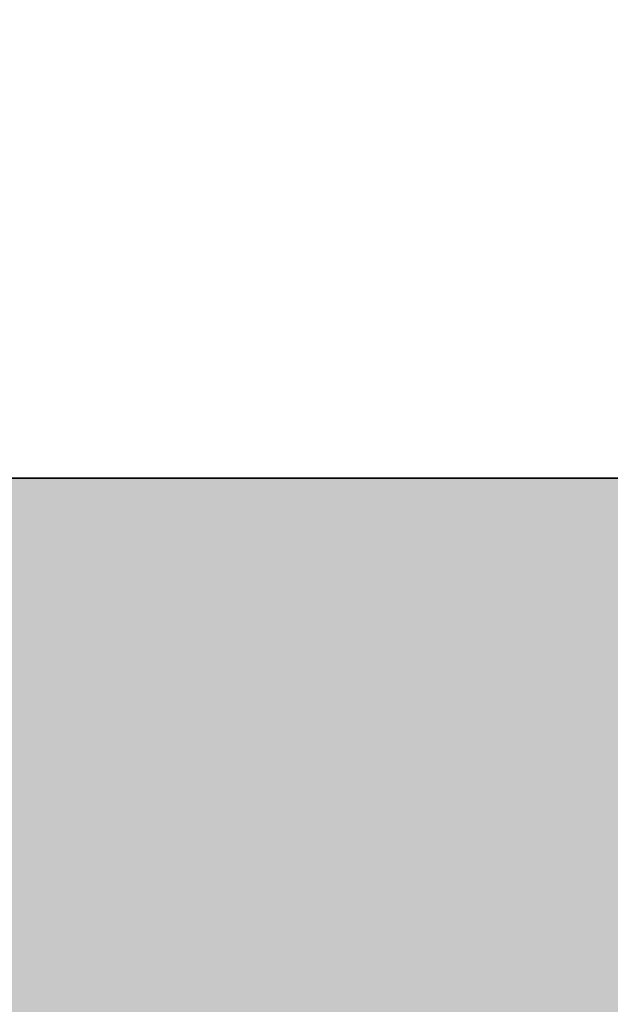
# Model space of a CAD drawing. Units: inches. Extents: x 2696 to 3240, y 1564 to 2310.
# Tile 70 of 76: x 3152.299 to 3156.715, y 2070.762 to 2078.132. Entities that reach past the tile are written whole.
import ezdxf

# ---------------------------------------------------------------- set-up
doc = ezdxf.new("R2010")
doc.units = ezdxf.units.IN
for name, color, linetype, lineweight in [('A-ANNO-DIMS', 3, 'Continuous', 18), ('A-WALL', 7, 'Continuous', 35), ('A-WALL-PATT', 9, 'Continuous', 13)]:
    doc.layers.add(name, color=color, linetype=linetype, lineweight=lineweight)
doc.styles.add('TIMES NEW', font='times.ttf')
doc.dimstyles.new('Siddhuu', dxfattribs={"dimtxt": 6, "dimasz": 2.5, "dimexe": 1.25, "dimexo": 0.625, "dimtad": 1, "dimdec": 1, "dimlunit": 4, "dimtxsty": 'TIMES NEW', "dimcen": 2.5, "dimclrd": 256, "dimclre": 1, "dimclrt": 7, "dimadec": 0, "dimazin": 0, "dimtfac": 1, "dimtdec": 1, "dimtmove": 0, "dimatfit": 3, "dimfxl": 1, "dimtolj": 1, "dimlwd": -1, "dimarcsym": 0})

# ---------------------------------------------------------------- blocks, each defined once
blk = doc.blocks.new('*D54')
at = {"layer": 'A-ANNO-DIMS', "color": 1, "lineweight": -2, "transparency": 16777216}
for p, q in [((3124.6114, 1893.8261), (3124.6114, 2298.4511)), ((3136.6114, 1893.8261), (3136.6114, 2298.4511))]:
    blk.add_line(p, q, dxfattribs=at)
at = {"layer": 'A-ANNO-DIMS', "transparency": 16777216}
for p, q in [((3127.1114, 2297.2011), (3134.1114, 2297.2011)), ((3136.6114, 2297.2011), (3155.7572, 2297.2011))]:
    blk.add_line(p, q, dxfattribs=at)
for points in [[(3127.1114, 2297.6178), (3127.1114, 2296.7844), (3124.6114, 2297.2011)], [(3134.1114, 2297.6178), (3134.1114, 2296.7844), (3136.6114, 2297.2011)]]:
    blk.add_solid(points, dxfattribs=at)
at = {"layer": 'Defpoints', "color": 0, "transparency": 16777216}
for p in [(3136.6114, 2297.2011), (3124.6114, 1893.2011), (3136.6114, 1893.2011)]:
    blk.add_point(p, dxfattribs=at)
at = {"layer": 'A-ANNO-DIMS', "color": 7, "transparency": 16777216, "insert": (3147.4343, 2300.878), "char_height": 6, "attachment_point": 5, "style": 'TIMES NEW'}
blk.add_mtext('\\A1;1\'-0"', dxfattribs=at)

msp = doc.modelspace()

# ---------------------------------------------------------------- hatches: boundary and pattern name
at = {"layer": 'A-WALL-PATT', "transparency": 33554556}
h = msp.add_hatch(color=256, dxfattribs=at)
h.dxf.hatch_style = 1
h.paths.add_polyline_path([(2879.1114, 2253.2011), (2905.9101, 2253.2011), (2905.9101, 2262.2011), (2841.889, 2262.2011), (2841.889, 2253.2011), (2870.1114, 2253.2011), (2870.1114, 2176.6011), (2965.7088, 2176.6011), (2965.7088, 2206.7011), (2973.5828, 2206.7011), (2973.5828, 2215.7011), (2965.7088, 2215.7011), (2965.7088, 2262.2011), (2929.9101, 2262.2011), (2929.9101, 2253.2011), (2956.7088, 2253.2011), (2956.7088, 2185.6011), (2879.1114, 2185.6011)])
h.paths.add_polyline_path([(2782.8338, 2262.2011), (2745.6114, 2262.2011), (2745.6114, 2228.7287), (2754.6114, 2228.7287), (2754.6114, 2253.2011), (2782.8338, 2253.2011)])
h.paths.add_polyline_path([(2754.6114, 2136.2011), (2965.7088, 2136.2011), (2965.7088, 2145.2011), (2879.1114, 2145.2011), (2879.1114, 2147.0735), (2877.3397, 2147.0735), (2870.1114, 2147.0735), (2870.1114, 2145.2011), (2754.6114, 2145.2011), (2754.6114, 2169.6735), (2745.6114, 2169.6735), (2745.6114, 2000.2011), (2754.6114, 2000.2011), (2754.6114, 2019.2011), (2849.0828, 2019.2011), (2849.0828, 2023.7011), (2841.2088, 2023.7011), (2841.2088, 2051.8271), (2836.7088, 2051.8271), (2836.7088, 2023.7011), (2754.6114, 2023.7011), (2754.6114, 2091.2011), (2836.7088, 2091.2011), (2836.7088, 2087.8271), (2841.2088, 2087.8271), (2841.2088, 2095.7011), (2754.6114, 2095.7011)])
h.paths.add_polyline_path([(2965.7088, 2136.2011), (2956.7088, 2136.2011), (2956.7088, 2023.7011), (2885.0828, 2023.7011), (2885.0828, 2019.2011), (2956.7088, 2019.2011), (2956.7088, 1950.5751), (2965.7088, 1950.5751), (2965.7088, 1980.2011), (2973.5828, 1980.2011), (2973.5828, 1989.2011), (2965.7088, 1989.2011)])
h.paths.add_polyline_path([(2754.6114, 1906.7011), (2880.2088, 1906.7011), (2884.7088, 1906.7011), (2956.7088, 1906.7011), (2956.7088, 1792.7011), (2944.7088, 1792.7011), (2944.7088, 1783.7011), (2956.7088, 1783.7011), (2956.7088, 1740.2011), (2884.7088, 1740.2011), (2884.7088, 1783.7011), (2896.7088, 1783.7011), (2896.7088, 1792.7011), (2884.7088, 1792.7011), (2884.7088, 1846.7011), (2880.2088, 1846.7011), (2880.2088, 1740.2011), (2754.6114, 1740.2011), (2754.6114, 1777.2011), (2745.6114, 1777.2011), (2745.6114, 1692.7011), (2754.6114, 1692.7011), (2754.6114, 1731.2011), (2956.7088, 1731.2011), (2956.7088, 1723.3271), (2965.7088, 1723.3271), (2965.7088, 1884.2011), (2973.5828, 1884.2011), (2973.5828, 1893.2011), (2965.7088, 1893.2011), (2965.7088, 1914.5751), (2956.7088, 1914.5751), (2956.7088, 1911.2011), (2754.6114, 1911.2011), (2754.6114, 1930.2011), (2745.6114, 1930.2011), (2745.6114, 1817.2011), (2754.6114, 1817.2011), (2754.6114, 1854.2011), (2826.6114, 1854.2011), (2826.6114, 1868.8271), (2822.1114, 1868.8271), (2822.1114, 1858.7011), (2754.6114, 1858.7011)])
h.paths.add_polyline_path([(2965.7088, 1656.2011), (3008.2374, 1656.2011), (3008.2374, 1665.2011), (2965.7088, 1665.2011), (2965.7088, 1693.3271), (2956.7088, 1693.3271), (2956.7088, 1686.2011), (2934.5828, 1686.2011), (2934.5828, 1681.7011), (2956.7088, 1681.7011), (2956.7088, 1614.2011), (2896.7088, 1614.2011), (2896.7088, 1681.7011), (2904.5828, 1681.7011), (2904.5828, 1686.2011), (2892.2088, 1686.2011), (2892.2088, 1614.2011), (2858.4101, 1614.2011), (2858.4101, 1605.2011), (2965.7088, 1605.2011)])
h.paths.add_polyline_path([(2788.4101, 1614.2011), (2754.6114, 1614.2011), (2754.6114, 1652.7011), (2745.6114, 1652.7011), (2745.6114, 1605.2011), (2788.4101, 1605.2011)])
h.paths.add_polyline_path([(3199.6114, 1633.0476), (3190.6114, 1633.0476), (3190.6114, 1614.2011), (3082.6114, 1614.2011), (3082.6114, 1665.2011), (3070.2374, 1665.2011), (3070.2374, 1656.2011), (3078.1114, 1656.2011), (3078.1114, 1605.2011), (3199.6114, 1605.2011)])
h.paths.add_polyline_path([(3199.6114, 1702.0476), (3190.6114, 1702.0476), (3190.6114, 1699.7011), (3106.6114, 1699.7011), (3106.6114, 1747.7011), (3190.6114, 1747.7011), (3190.6114, 1752.2011), (3082.6114, 1752.2011), (3082.6114, 1760.0751), (3078.1114, 1760.0751), (3078.1114, 1747.7011), (3102.1114, 1747.7011), (3102.1114, 1699.7011), (3078.1114, 1699.7011), (3078.1114, 1695.2011), (3190.6114, 1695.2011), (3190.6114, 1676.3546), (3199.6114, 1676.3546)])
h.paths.add_polyline_path([(3199.6114, 1783.2011), (3190.6114, 1783.2011), (3190.6114, 1745.3546), (3199.6114, 1745.3546)])
h.paths.add_polyline_path([(3082.6114, 1884.2011), (3190.6114, 1884.2011), (3190.6114, 1853.2011), (3199.6114, 1853.2011), (3199.6114, 1901.7011), (3190.6114, 1901.7011), (3190.6114, 1893.2011), (3005.5828, 1893.2011), (3005.5828, 1891.2811), (3005.5828, 1884.2011), (3078.1114, 1884.2011), (3078.1114, 1792.0751), (3082.6114, 1792.0751)])
h.paths.add_polyline_path([(3199.6114, 1994.7011), (3190.6114, 1994.7011), (3190.6114, 1989.2011), (3073.7088, 1989.2011), (3073.7088, 2034.2011), (3069.2088, 2034.2011), (3069.2088, 1989.2011), (3005.5828, 1989.2011), (3005.5828, 1980.2011), (3190.6114, 1980.2011), (3190.6114, 1971.7011), (3199.6114, 1971.7011)])
h.paths.add_polyline_path([(3199.6114, 2155.2011), (3190.6114, 2155.2011), (3190.6114, 2064.7011), (3199.6114, 2064.7011)])
h.paths.add_polyline_path([(3190.6114, 2074.7011), (3106.6114, 2074.7011), (3106.6114, 2122.7011), (3190.6114, 2122.7011), (3190.6114, 2127.2011), (3082.7088, 2127.2011), (3082.7088, 2135.0751), (3073.7088, 2135.0751), (3073.7088, 2122.7011), (3102.1114, 2122.7011), (3102.1114, 2074.7011), (3069.2088, 2074.7011), (3069.2088, 2070.2011), (3190.6114, 2070.2011)])
h.paths.add_polyline_path([(3082.7088, 2253.2011), (3190.6114, 2253.2011), (3190.6114, 2225.2011), (3199.6114, 2225.2011), (3199.6114, 2262.2011), (3073.7088, 2262.2011), (3073.7088, 2215.7011), (3035.5828, 2215.7011), (3035.5828, 2206.7011), (3073.7088, 2206.7011), (3073.7088, 2171.0751), (3082.7088, 2171.0751)])

# ---------------------------------------------------------------- linework, layer by layer
at = {"layer": 'A-WALL'}
msp.add_line((3106.6114, 2074.7011), (3190.6114, 2074.7011), dxfattribs=at)

# ---------------------------------------------------------------- dimensions: what is measured, and where the dimension line sits
at = {"layer": 'A-ANNO-DIMS'}
dim = msp.add_linear_dim(base=(3136.6114, 2297.2011), p1=(3124.6114, 1893.2011), p2=(3136.6114, 1893.2011), dimstyle='Siddhuu', override={"dimdec": 1, "dimlfac": 1, "dimrnd": 0, "dimzin": 1, "dimdsep": 46, "dimlunit": 4, "dimfrac": 2}, dxfattribs=at)
dim.commit()
dim.dimension.update_dxf_attribs({"geometry": '*D54', "text_midpoint": (3147.4343, 2300.878)})

doc.saveas('drawing.dxf')
